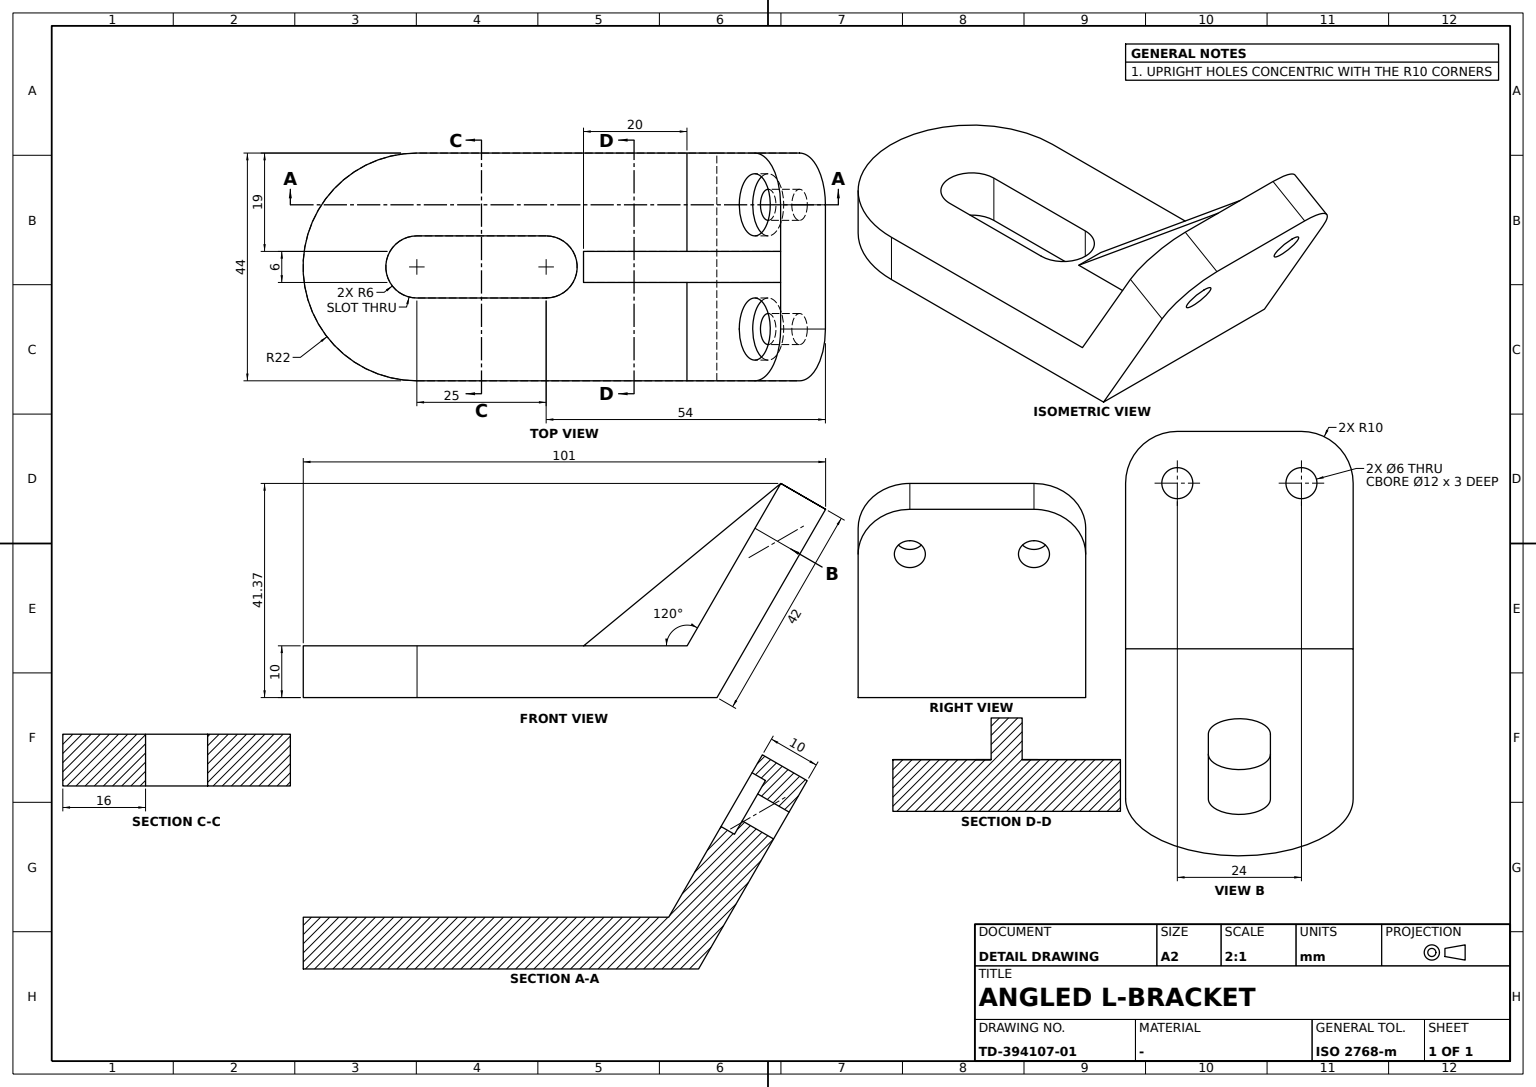
CATIA V5 part; units mm, degrees
sketch "Sketch1" plane through (0, 0, 0) normal (0, 0, 1) x (1, 0, 0)
  line L0 (58, 22) -> (0, 22)
  point P0 (0, 22)
  line L1 (0, 22) -> (0, -22)
  line L2 (0, -22) -> (58, -22)
  arc A0 (58, -22) -> (58, 22) centre (58, 0) ccw
  arc A1 (58, -6) -> (58, 6) centre (58, 0) ccw
  arc A2 (33, 6) -> (33, -6) centre (33, 0) ccw
  line L3 (33, 6) -> (58, 6)
  line L4 (33, -6) -> (58, -6)
  dimension "length L1" = 44
  dimension "radius A1" = 6
  dimension "radius A2" = 6
  constraint coincidence P0 y-axis
  constraint horizontal L0 x-axis
  constraint horizontal L2 x-axis
  constraint vertical L1 y-axis
  constraint tangency A0 L0
  constraint tangency L3 A2
  constraint tangency L3 A1
  constraint tangency L4 A2
  constraint tangency L4 A1
extrude "Pad1" add sketch "Sketch1" along normal blind 10
sketch "Sketch2" plane through (0, -22, 0) normal (0, -1, 0) x (1, 0, 0)
  line L0 (0, 0) -> (-21, 36.3731)
  line L1 (-21, 36.3731) -> (-12.3397, 41.3731)
  line L2 (-12.3397, 41.3731) -> (5.7735, 10)
  point P0 (5.7735, 10)
  line L3 (0, 0) -> (5.7735, 10)
  point P1 (0, 0)
  point P2 (5.7735, 10)
  dimension "length L0" = 42
  dimension "angle L0 x axis" = 120
  dimension "length L1" = 10
  constraint parallelism L2 L0
  constraint coincidence P1 L0
  constraint coincidence P1 y-axis
  constraint coincidence L3 P0
  constraint coincidence origin P1
  constraint coincidence P0 P2
extrude "Pad2" add sketch "Sketch2" against normal blind 44
fillet "Fillet1" radius 10 2 edges at (-16.6699, -22, 38.8731) (-16.6699, 22, 38.8731)
sketch "Sketch4" plane through (8.6603, 0, 5) normal (0.866, 0, 0.5) x (0, 1, 0)
  circle A0 centre (12, 32) radius 6
  circle A1 centre (-12, 32) radius 6
  dimension "radius A0" = 6
  constraint symmetry A0 A1 y-axis
extrude "Pocket1" cut sketch "Sketch4" against normal blind 3
sketch "Sketch5" plane through (6.0622, 0, 3.5) normal (0.866, 0, 0.5) x (0, 1, 0)
  circle A0 centre (12, 32) radius 3
  circle A1 centre (-12, 32) radius 3
  dimension "radius A0" = 3
  constraint symmetry A0 A1 y-axis
extrude "Pocket2" cut sketch "Sketch5" against normal through all
sketch "Sketch6" plane through (0, 0, 0) normal (0, 1, 0) x (-1, 0, 0)
  point P0 (-5.7735, 10)
  line L0 (12.3397, 41.3731) -> (-25.7735, 10)
  point P1 (-25.7735, 10)
  dimension "distance P1 P0" = 20
rib "Stiffener1" sketch "Sketch6" thickness 6 sides both
sketch "Sketch3" plane through (8.6603, 0, 5) normal (0.866, 0, 0.5) x (0, 1, 0)
